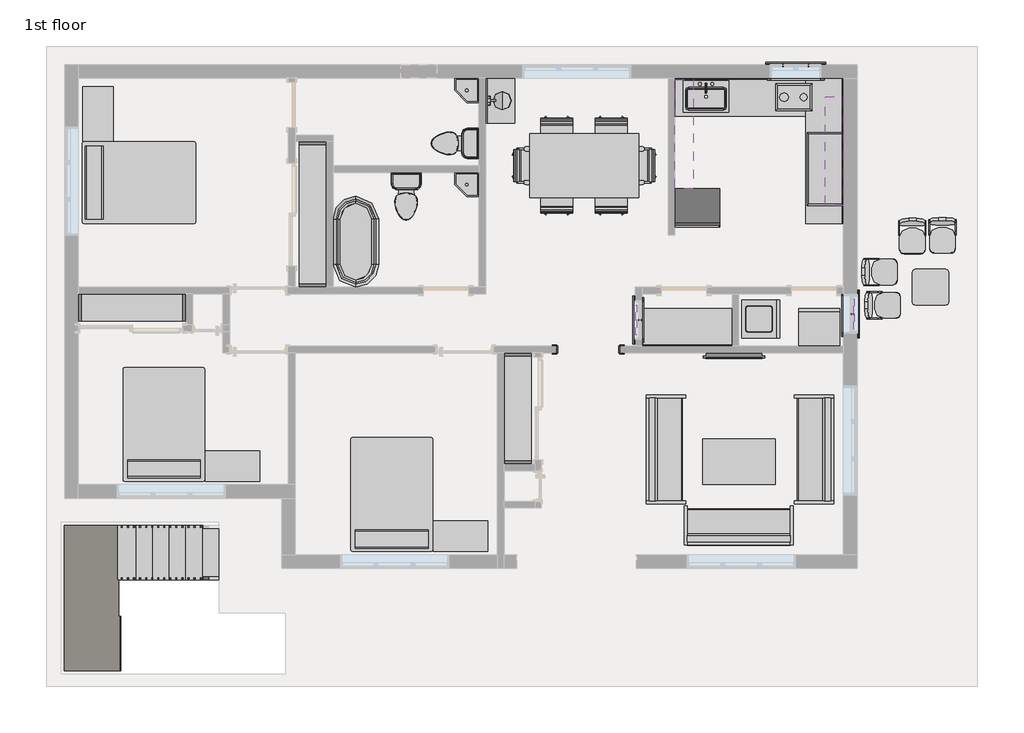
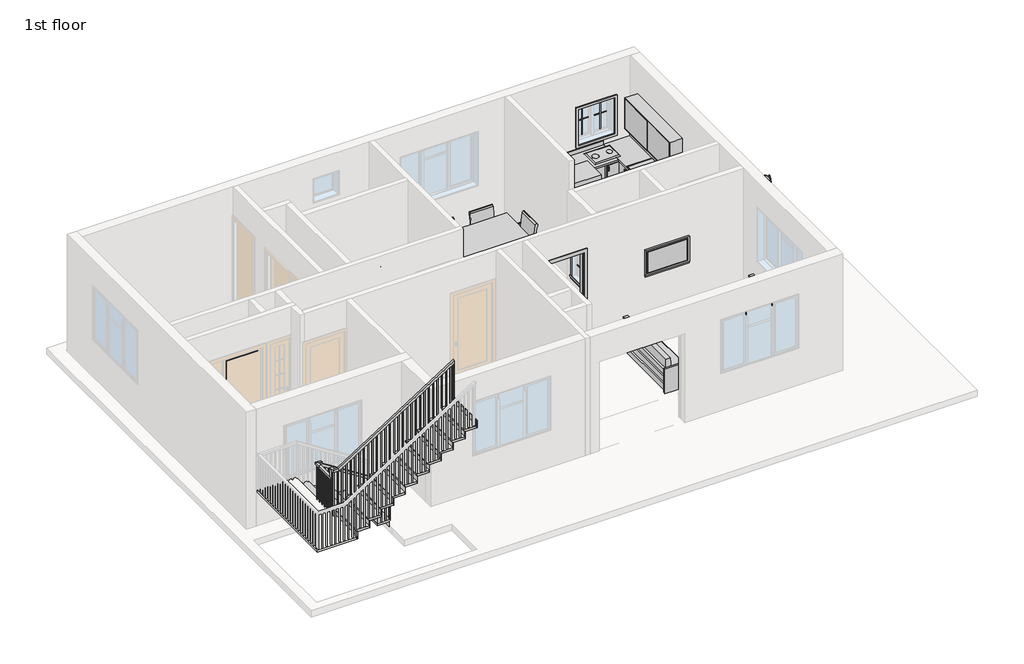
# One storey, part 4 of 4: 34 furniture elements, 17 proxies, 7 flow terminals, 2 stair flights, 1 railing, 1 slab.
# Revit data of these elements (continued)
# Type "Handrail - Rectangular" (continued)
#   built-in parameter 1008611 = 0.0416667 (stored number, unit not read)
#   built-in parameter 1008609 = 0.333333 (stored number, unit not read)
#   built-in parameter 1008604 = 0.166667 (stored number, unit not read)
#   built-in parameter 1008603 = 0.166667 (stored number, unit not read)
#   Railing Height = 3' - 0"
#   built-in parameter 1008630 = 2
#   built-in parameter 1008610 = 2
#   built-in parameter 1008618 = Baluster - Square : 3/4"
# Element 1 (IfcBuildingElementProxy, "Cook Top-2 Unit : 12\" x 18\"")
#   Phase Created = New Construction
#   Materials on its faces: "Metal - Steel, Polished", "Metal - Chrome"
# Element 2 (IfcBuildingElementProxy, "Dryer : 27\" x 25\" x 35\"")
#   Phase Created = New Construction
#   Materials on its faces: "Metal - Paint Finish - Ivory,Glossy"
# Elements 3, 4 (IfcBuildingElementProxy, "Muntin Pattern_2x2 : Muntin Pattern_2x2")
#   Width = 0' - 11 5/8"
#   Height = 2' - 6 1/2"
#   Interior Material = Wood - Stained
#   Exterior Material = Clad - White
#   Phase Created = New Construction
#   Materials on its faces: "Clad - White", "Wood - Stained"
# Elements 5, 6, 7, 8 (IfcBuildingElementProxy, "Muntin Pattern_2x2 : Muntin Pattern_2x2")
#   Width = 1' - 8"
#   Height = 1' - 5 1/8"
#   Interior Material = Wood - Stained
#   Exterior Material = Clad - White
#   Phase Created = New Construction
#   Materials on its faces: "Clad - White", "Wood - Stained"
# Element 9 (IfcBuildingElementProxy, "Passage Opening-Cased : 36\" x 84\"")
#   Phase Created = New Construction
#   Materials on its faces: "Door - Frame"
# Element 10 (IfcBuildingElementProxy, "Refrigerator-Built-in : 30\" x 24\" RH")
#   Phase Created = New Construction
#   Materials on its faces: "Metal - Paint Finish - Ivory,Glossy", "Metal - Chrome"
# Element 11 (IfcBuildingElementProxy, "Trim-Window-Exterior-Flat : with Sill")
#   Opening Width = 2' - 10"
#   Opening Height = 3' - 0"
#   Trim Material = Clad - White
#   Phase Created = New Construction
#   Materials on its faces: "Clad - White"
# Elements 12, 13 (IfcBuildingElementProxy, "Trim-Window-Exterior-Flat : with Sill")
#   Opening Width = 2' - 2"
#   Opening Height = 3' - 6"
#   Trim Material = Clad - White
#   Phase Created = New Construction
#   Materials on its faces: "Clad - White"
# Element 14 (IfcBuildingElementProxy, "Trim-Window-Interior-Flat : Picture Frame")
#   Opening Width = 2' - 10"
#   Opening Height = 3' - 0"
#   Trim Material = Wood - Stained
#   Phase Created = New Construction
#   Materials on its faces: "Wood - Stained"
# Elements 15, 16 (IfcBuildingElementProxy, "Trim-Window-Interior-Flat : Picture Frame")
#   Opening Width = 2' - 2"
#   Opening Height = 3' - 6"
#   Trim Material = Wood - Stained
#   Phase Created = New Construction
#   Materials on its faces: "Wood - Stained"
# Element 17 (IfcBuildingElementProxy, "Washer : 25\" x 25\" x 35\"")
#   Phase Created = New Construction
#   Materials on its faces: "Metal - Paint Finish - Ivory,Matte"
# Element 18 (IfcFlowTerminal, "Lavatory - Vanity : 30\"x18\" - Private")
#   Mark = "13"
#   Flow Pressure = 8.00 psi
#   Phase Created = New Construction
# Element 19 (IfcFlowTerminal, "Sink - Mop : 28\"x28\"")
#   Mark = "11"
#   Phase Created = New Construction
# Element 20 (IfcFlowTerminal, "Sink - Mop : 28\"x28\"")
#   Mark = "12"
#   Phase Created = New Construction
# Element 21 (IfcFlowTerminal, "Sink Kitchen-Single : 30\" x 21\"")
#   Mark = "10"
#   Phase Created = New Construction
#   Materials on its faces: "Steel, Polished"
# Element 22 (IfcFlowTerminal, "Toilet-Domestic-3D : Toilet-Domestic-3D")
#   Mark = "14"
#   Phase Created = New Construction
#   Materials on its faces: "Porcelain, Linen", "Laminate, Linen, Matte"
# Element 23 (IfcFlowTerminal, "Toilet-Domestic-3D : Toilet-Domestic-3D")
#   Mark = "15"
#   Phase Created = New Construction
#   Materials on its faces: "Porcelain, Linen", "Laminate, Linen, Matte"
# Element 24 (IfcFlowTerminal, "Tub-Free Standing-3D : 30\" x 60\"")
#   Mark = "9"
#   Phase Created = New Construction
#   Materials on its faces: "Porcelain, Ivory"
# Element 25 (IfcFurniture, "48\"")
#   Phase Created = New Construction
#   Materials on its faces: "Cabinets", "Cabinets - Handles"
# Element 26 (IfcFurniture, "Base Cabinet-Combo01 : 30\"")
#   Phase Created = New Construction
#   Materials on its faces: "Cabinet"
# Element 27 (IfcFurniture, "Base Cabinet-Corner Unit-Square : 36\"")
#   Phase Created = New Construction
#   Materials on its faces: "Cabinets", "Cabinets - Handles"
# Elements 28, 29, 30 (IfcFurniture, "Bed-Standard : Double 54\" x 75\"")
#   Phase Created = New Construction
#   Materials on its faces: "Linen, White", "Steel, Chrome Plated"
# Elements 31, 32, 33 (IfcFurniture, "Cabinet File-Lateral 2 Drawer : 36\" x 20\" x 24\"")
#   Phase Created = New Construction
#   Materials on its faces: "Metal - Steel"
# Elements 34, 35, 36, 37 (IfcFurniture, "Chair-Task : Chair-Task")
#   Phase Created = New Construction
#   Materials on its faces: "Plastic - Black", "Textile - Slate Blue"
# Elements 38, 39 (IfcFurniture, "Chair-Task Arms : Chair-Task Arms")
#   Phase Created = New Construction
#   Materials on its faces: "Plastic - Black", "Textile - Slate Blue"
# Element 40 (IfcFurniture, "Counter Top : 24\" Depth")
#   Length = 8' - 0"
#   Phase Created = New Construction
#   Materials on its faces: "Counter Top"
# Element 41 (IfcFurniture, "Counter Top : 24\" Depth")
#   Length = 4' - 11 1/2"
#   Phase Created = New Construction
#   Materials on its faces: "Counter Top"
# Element 42 (IfcFurniture, "Counter Top w Sink Hole : 24\" Depth")
#   Sink Opening Width = 2' - 3"
#   Sink Opening Depth = 1' - 3"
#   Sink Location To Wall = 0' - 6"
#   Sink Location = 1' - 8 1/2"
#   Length = 7' - 2 1/4"
#   Phase Created = New Construction
#   Materials on its faces: "Counter Top"
# Elements 43, 44, 45, 46 (IfcFurniture, "Seating-Auditorium : 18\" x 24\" x 30\"")
#   Phase Created = New Construction
#   Materials on its faces: "Steel, Paint Finish, Dark Gray, Matte", "Linen, Beige"
# Element 47 (IfcFurniture, "Shelving : 96\" x 12\" x 84\"")
#   Phase Created = New Construction
#   Materials on its faces: "Laminate, Ivory, Matte"
# Element 48 (IfcFurniture, "Shelving : 96\" x 12\" x 84\" 2")
#   Phase Created = New Construction
#   Materials on its faces: "Laminate, Ivory, Matte"
# Element 49 (IfcFurniture, "Shelving : 96\" x 12\" x 84\" 3")
#   Phase Created = New Construction
#   Materials on its faces: "Laminate, Ivory, Matte"
# Elements 50, 51, 52 (IfcFurniture, "Sofa : 72\"")
#   Phase Created = New Construction
#   Materials on its faces: "Cherry", "Linen, Beige"
# Element 53 (IfcFurniture, "Table-Coffee Rectangular : 48\" x 30\"")
#   Phase Created = New Construction
#   Materials on its faces: "Metal - Chrome", "Glass - Clear, Grey"
# Element 54 (IfcFurniture, "Table-Conference2 w Chairs : 40\" x 90\"")
#   Phase Created = New Construction
#   Materials on its faces: "Wood - Cherry"
# Element 55 (IfcFurniture, "Table-End : 24\" x 24\"")
#   Phase Created = New Construction
#   Materials on its faces: "Laminate, Ivory, Matte", "Birch"
# Element 56 (IfcFurniture, "Television-Plasma : 42\"")
#   Phase Created = New Construction
#   Materials on its faces: "Plastic - Gray", "Glass"
# Elements 57, 58 (IfcFurniture, "Upper Cabinet-Pass-Thru w Glass : 48\" x 30\" x 12\"")
#   Phase Created = New Construction
#   Materials on its faces: "Glass", "Cabinet"
# Element 59 (IfcRailing, "Handrail - Rectangular")
#   Phase Created = New Construction
# Element 60 (IfcSlab, "Non-Monolithic Landing")
#   Phase Created = New Construction
# Elements 61, 62 (IfcStairFlight, "2\" Tread 1\" Nosing 1/4\" Riser")
#   Phase Created = New Construction
# Materials
#   "Metal - Chrome": colour RGB 57 57 57, transparency 0
#   "Metal - Steel, Polished": colour RGB 57 57 57, transparency 0
#   "Metal - Paint Finish - Ivory,Glossy": colour RGB 247 247 239, transparency 0
#   "Door - Frame": colour RGB 118 70 51, transparency 0, Cost = 0
#   "Metal - Paint Finish - Ivory,Matte": colour RGB 247 247 239, transparency 0
#   "Steel, Polished": class "Metal", colour RGB 57 57 57, transparency 0, Description = "Polished steel", Cost = 0
#   "Porcelain, Linen": class "Ceramic", colour RGB 249 239 230, transparency 0, Description = "Porcelain, linen", Cost = 0
#   "Laminate, Linen, Matte": class "Plastic", colour RGB 249 239 230, transparency 0, Description = "Plastic Laminate - Linen, Matte", Cost = 0
#   "Porcelain, Ivory": class "Ceramic", colour RGB 247 247 239, transparency 0, Description = "Porcelain, ivory", Cost = 0
#   "Cabinets - Handles": class "Metal", colour RGB 57 57 57, transparency 0
#   "Cabinets": colour RGB 249 249 249, transparency 0
#   "Steel, Chrome Plated": class "Metal", colour RGB 17 17 17, transparency 0, Description = "Chromiuim plated steel", Cost = 0
#   "Linen, White": class "Textile", colour RGB 247 247 239, transparency 0, Description = "Linen, white", Cost = 0
#   "Metal - Steel": colour RGB 210 210 210, transparency 0
#   "Plastic - Black": colour RGB 0 0 0, transparency 0
#   "Textile - Slate Blue": colour RGB 98 102 118, transparency 0
#   "Linen, Beige": class "Textile", colour RGB 249 239 230, transparency 0, Description = "Linen, beige", Cost = 0
#   "Steel, Paint Finish, Dark Gray, Matte": class "Metal", colour RGB 0 0 0, transparency 0, Description = "Steel, paint finish, dark gray, matte", Cost = 0
#   "Laminate, Ivory, Matte": class "Plastic", colour RGB 247 247 239, transparency 0, Description = "Plastic Laminate - Ivory, Matte", Cost = 0
#   "Cherry": class "Wood", colour RGB 226 177 128, transparency 0, Description = "Prunus Serotina", Cost = 0
#   "Glass - Clear, Grey": colour RGB 252 255 255, transparency 0.64
#   "Wood - Cherry": colour RGB 151 75 0, transparency 0
#   "Birch": class "Wood", colour RGB 224 178 126, transparency 0, Description = "Betula Alleghaniensis", Cost = 0
#   "Plastic - Gray": colour RGB 134 134 134, transparency 0
#   "Clad - White": class "Wood", colour RGB 242 242 238, transparency 0, Cost = 0
#   "Wood - Stained": class "Wood", colour RGB 224 178 126, transparency 0, Cost = 0
#   "Cabinet": colour RGB 204 122 2, transparency 0
#   "Counter Top": class "Wood", colour RGB 226 177 128, transparency 0
#   "Glass": class "Glass", colour RGB 0 128 192, transparency 0.75, Description = "Soda Lime Glass", Cost = 0
